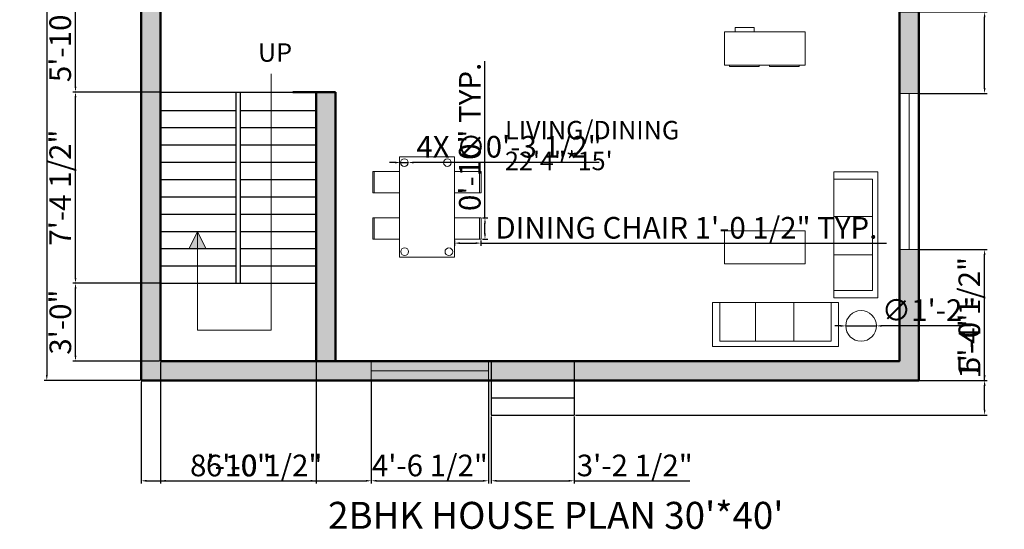
# Model space of a CAD drawing. Units: inches. Extents: x 1369 to 1956, y 3714 to 4363.
# Tile 1 of 2: x 1369 to 1825, y 3714 to 3949. Entities that reach past the tile are written whole.
import ezdxf

# ---------------------------------------------------------------- set-up
doc = ezdxf.new("R2010")
doc.units = ezdxf.units.IN
for name, color, linetype, lineweight in [('A-ANNO-DIMS', 2, 'Continuous', 18), ('A-ANNO-SYMB', 7, 'Continuous', 18), ('A-ANNO-TEXT', 7, 'Continuous', 25), ('A-AREA-IDEN', 7, 'Continuous', 25), ('A-FLOR-STRS', 7, 'Continuous', 25), ('A-FURN', 8, 'Continuous', 18), ('A-GLAZ', 4, 'Continuous', 18), ('A-WALL', 7, 'Continuous', 50), ('A-WALL-PATT', 252, 'Continuous', 13)]:
    doc.layers.add(name, color=color, linetype=linetype, lineweight=lineweight)
doc.styles.get("Standard").update_dxf_attribs({"font": 'arial.ttf'})
doc.dimstyles.new('ISO-25', dxfattribs={"dimtxt": 10, "dimasz": 2.5, "dimexe": 1.25, "dimexo": 0.625, "dimtad": 1, "dimdec": 0, "dimlunit": 4, "dimtxsty": 'Standard', "dimcen": 2.5, "dimadec": 0, "dimazin": 0, "dimtfac": 1, "dimtdec": 0, "dimtmove": 0, "dimatfit": 3, "dimfxl": 1, "dimarcsym": 0})

# ---------------------------------------------------------------- blocks, each defined once
blk = doc.blocks.new('*D6')
at = {"layer": 'A-ANNO-DIMS', "color": 0, "lineweight": -2, "transparency": 16777216}
for p, q in [((1424.56, 4262.45), (1380.24, 4262.45)), ((1381.49, 4259.95), (1381.49, 3784.95)), ((1424.56, 3782.45), (1380.24, 3782.45))]:
    blk.add_line(p, q, dxfattribs=at)
at = {"layer": 'A-ANNO-DIMS', "color": 0, "transparency": 16777216}
for points in [[(1381.07, 4259.95), (1381.9, 4259.95), (1381.49, 4262.45)], [(1381.07, 3784.95), (1381.9, 3784.95), (1381.49, 3782.45)]]:
    blk.add_solid(points, dxfattribs=at)
at = {"layer": 'Defpoints', "color": 0, "transparency": 16777216}
for p in [(1425.18, 4262.45), (1381.49, 3782.45), (1425.18, 3782.45)]:
    blk.add_point(p, dxfattribs=at)
at = {"layer": 'A-ANNO-DIMS', "color": 0, "transparency": 16777216, "insert": (1375.76, 4022.45), "char_height": 10, "attachment_point": 5, "rotation": 90}
blk.add_mtext("40'", dxfattribs=at)
blk = doc.blocks.new('WINDOW-72IN')
blk.add_line((0, 4.5), (72.22, 4.5))
blk.add_lwpolyline([(0, 9), (72.22, 9), (72.22, 0), (0, 0)], close=True)
blk = doc.blocks.new('CHAIR-DINING')
blk.add_line((11.59, 9.82), (11.59, 0))
blk.add_lwpolyline([(0, 9.82), (12.29, 9.82), (12.29, 0), (0, 0)], close=True)
blk = doc.blocks.new('*D12')
at = {"layer": 'A-ANNO-DIMS', "color": 0, "lineweight": -2, "transparency": 16777216}
for p, q in [((1570.19, 3847.22), (1570.19, 3844.76)), ((1582.47, 3847.22), (1582.47, 3844.76)), ((1572.69, 3846.01), (1579.97, 3846.01)), ((1582.47, 3846.01), (1770.1, 3846.01))]:
    blk.add_line(p, q, dxfattribs=at)
at = {"layer": 'A-ANNO-DIMS', "color": 0, "transparency": 16777216}
for points in [[(1572.69, 3846.42), (1572.69, 3845.59), (1570.19, 3846.01)], [(1579.97, 3846.42), (1579.97, 3845.59), (1582.47, 3846.01)]]:
    blk.add_solid(points, dxfattribs=at)
at = {"layer": 'Defpoints', "color": 0, "transparency": 16777216}
for p in [(1570.19, 3847.85), (1582.47, 3847.85), (1582.47, 3846.01)]:
    blk.add_point(p, dxfattribs=at)
at = {"layer": 'A-ANNO-DIMS', "color": 0, "transparency": 16777216, "insert": (1677.54, 3851.8), "char_height": 10, "attachment_point": 5}
blk.add_mtext('DINING CHAIR 1\'-0 1/2" TYP.', dxfattribs=at)
blk = doc.blocks.new('*D13')
at = {"layer": 'A-ANNO-DIMS', "color": 0, "lineweight": -2, "transparency": 16777216}
for p, q in [((1584.31, 3857.67), (1584.31, 3930.14)), ((1583.1, 3857.67), (1585.56, 3857.67)), ((1584.31, 3850.35), (1584.31, 3855.17)), ((1583.1, 3847.85), (1585.56, 3847.85))]:
    blk.add_line(p, q, dxfattribs=at)
at = {"layer": 'A-ANNO-DIMS', "color": 0, "transparency": 16777216}
for points in [[(1583.9, 3855.17), (1584.73, 3855.17), (1584.31, 3857.67)], [(1583.9, 3850.35), (1584.73, 3850.35), (1584.31, 3847.85)]]:
    blk.add_solid(points, dxfattribs=at)
at = {"layer": 'Defpoints', "color": 0, "transparency": 16777216}
for p in [(1582.47, 3857.67), (1584.31, 3857.67), (1582.47, 3847.85)]:
    blk.add_point(p, dxfattribs=at)
at = {"layer": 'A-ANNO-DIMS', "color": 0, "transparency": 16777216, "insert": (1578.58, 3895.16), "char_height": 10, "attachment_point": 5, "rotation": 90}
blk.add_mtext('0\'-10" TYP.', dxfattribs=at)
blk = doc.blocks.new('*D16')
at = {"layer": 'A-ANNO-DIMS', "color": 0, "lineweight": -2, "transparency": 16777216}
for p, q in [((1434.18, 3790.82), (1434.18, 3734.8)), ((1506.18, 3790.82), (1506.18, 3734.8)), ((1436.68, 3736.05), (1503.68, 3736.05))]:
    blk.add_line(p, q, dxfattribs=at)
at = {"layer": 'A-ANNO-DIMS', "color": 0, "transparency": 16777216}
for points in [[(1436.68, 3736.46), (1436.68, 3735.63), (1434.18, 3736.05)], [(1503.68, 3736.46), (1503.68, 3735.63), (1506.18, 3736.05)]]:
    blk.add_solid(points, dxfattribs=at)
at = {"layer": 'Defpoints', "color": 0, "transparency": 16777216}
for p in [(1434.18, 3791.45), (1506.18, 3791.45), (1506.18, 3736.05)]:
    blk.add_point(p, dxfattribs=at)
at = {"layer": 'A-ANNO-DIMS', "color": 0, "transparency": 16777216, "insert": (1470.18, 3741.78), "char_height": 10, "attachment_point": 5}
blk.add_mtext('6\'-0"', dxfattribs=at)
blk = doc.blocks.new('*D17')
at = {"layer": 'A-ANNO-DIMS', "color": 0, "lineweight": -2, "transparency": 16777216}
for p, q in [((1433.56, 3827.45), (1393.53, 3827.45)), ((1394.78, 3793.95), (1394.78, 3824.95)), ((1433.56, 3791.45), (1393.53, 3791.45))]:
    blk.add_line(p, q, dxfattribs=at)
at = {"layer": 'A-ANNO-DIMS', "color": 0, "transparency": 16777216}
for points in [[(1394.36, 3824.95), (1395.2, 3824.95), (1394.78, 3827.45)], [(1394.36, 3793.95), (1395.2, 3793.95), (1394.78, 3791.45)]]:
    blk.add_solid(points, dxfattribs=at)
at = {"layer": 'Defpoints', "color": 0, "transparency": 16777216}
for p in [(1394.78, 3827.45), (1434.18, 3827.45), (1434.18, 3791.45)]:
    blk.add_point(p, dxfattribs=at)
at = {"layer": 'A-ANNO-DIMS', "color": 0, "transparency": 16777216, "insert": (1389.05, 3809.45), "char_height": 10, "attachment_point": 5, "rotation": 90}
blk.add_mtext('3\'-0"', dxfattribs=at)
blk = doc.blocks.new('*D18')
at = {"layer": 'A-ANNO-DIMS', "color": 0, "lineweight": -2, "transparency": 16777216}
for p, q in [((1433.56, 3915.93), (1393.53, 3915.93)), ((1394.78, 3829.95), (1394.78, 3913.43)), ((1433.56, 3827.45), (1393.53, 3827.45))]:
    blk.add_line(p, q, dxfattribs=at)
at = {"layer": 'A-ANNO-DIMS', "color": 0, "transparency": 16777216}
for points in [[(1394.36, 3913.43), (1395.2, 3913.43), (1394.78, 3915.93)], [(1394.36, 3829.95), (1395.2, 3829.95), (1394.78, 3827.45)]]:
    blk.add_solid(points, dxfattribs=at)
at = {"layer": 'Defpoints', "color": 0, "transparency": 16777216}
for p in [(1394.78, 3915.93), (1434.18, 3915.93), (1434.18, 3827.45)]:
    blk.add_point(p, dxfattribs=at)
at = {"layer": 'A-ANNO-DIMS', "color": 0, "transparency": 16777216, "insert": (1388.99, 3871.69), "char_height": 10, "attachment_point": 5, "rotation": 90}
blk.add_mtext('7\'-4 1/2"', dxfattribs=at)
blk = doc.blocks.new('*D19')
at = {"layer": 'A-ANNO-DIMS', "color": 0, "lineweight": -2, "transparency": 16777216}
for p, q in [((1587.22, 3765.82), (1587.22, 3734.8)), ((1625.58, 3765.82), (1625.58, 3734.8)), ((1589.72, 3736.05), (1623.08, 3736.05)), ((1625.58, 3736.05), (1679.2, 3736.05))]:
    blk.add_line(p, q, dxfattribs=at)
at = {"layer": 'A-ANNO-DIMS', "color": 0, "transparency": 16777216}
for points in [[(1589.72, 3736.46), (1589.72, 3735.63), (1587.22, 3736.05)], [(1623.08, 3736.46), (1623.08, 3735.63), (1625.58, 3736.05)]]:
    blk.add_solid(points, dxfattribs=at)
at = {"layer": 'Defpoints', "color": 0, "transparency": 16777216}
for p in [(1587.22, 3766.45), (1625.58, 3766.45), (1625.58, 3736.05)]:
    blk.add_point(p, dxfattribs=at)
at = {"layer": 'A-ANNO-DIMS', "color": 0, "transparency": 16777216, "insert": (1653.64, 3741.85), "char_height": 10, "attachment_point": 5}
blk.add_mtext('3\'-2 1/2"', dxfattribs=at)
blk = doc.blocks.new('*D20')
at = {"layer": 'A-ANNO-DIMS', "color": 0, "lineweight": -2, "transparency": 16777216}
for p, q in [((1815.58, 3782.45), (1815.58, 3811.84)), ((1626.2, 3782.45), (1816.83, 3782.45)), ((1815.58, 3768.95), (1815.58, 3779.95)), ((1626.2, 3766.45), (1816.83, 3766.45))]:
    blk.add_line(p, q, dxfattribs=at)
at = {"layer": 'A-ANNO-DIMS', "color": 0, "transparency": 16777216}
for points in [[(1815.16, 3779.95), (1816, 3779.95), (1815.58, 3782.45)], [(1815.16, 3768.95), (1816, 3768.95), (1815.58, 3766.45)]]:
    blk.add_solid(points, dxfattribs=at)
at = {"layer": 'Defpoints', "color": 0, "transparency": 16777216}
for p in [(1625.58, 3782.45), (1815.58, 3782.45), (1625.58, 3766.45)]:
    blk.add_point(p, dxfattribs=at)
at = {"layer": 'A-ANNO-DIMS', "color": 0, "transparency": 16777216, "insert": (1809.94, 3798.39), "char_height": 10, "attachment_point": 5, "rotation": 90}
blk.add_mtext('1\'-4"', dxfattribs=at)
blk = doc.blocks.new('*D23')
at = {"layer": 'A-ANNO-DIMS', "color": 0, "lineweight": -2, "transparency": 16777216}
for p, q in [((1425.18, 3781.82), (1425.18, 3734.8)), ((1531.68, 3781.82), (1531.68, 3734.8)), ((1427.68, 3736.05), (1529.18, 3736.05))]:
    blk.add_line(p, q, dxfattribs=at)
at = {"layer": 'A-ANNO-DIMS', "color": 0, "transparency": 16777216}
for points in [[(1427.68, 3736.46), (1427.68, 3735.63), (1425.18, 3736.05)], [(1529.18, 3736.46), (1529.18, 3735.63), (1531.68, 3736.05)]]:
    blk.add_solid(points, dxfattribs=at)
at = {"layer": 'Defpoints', "color": 0, "transparency": 16777216}
for p in [(1425.18, 3782.45), (1531.68, 3782.45), (1531.68, 3736.05)]:
    blk.add_point(p, dxfattribs=at)
at = {"layer": 'A-ANNO-DIMS', "color": 0, "transparency": 16777216, "insert": (1478.43, 3741.84), "char_height": 10, "attachment_point": 5}
blk.add_mtext('8\'-10 1/2"', dxfattribs=at)
blk = doc.blocks.new('*D24')
at = {"layer": 'A-ANNO-DIMS', "color": 0, "lineweight": -2, "transparency": 16777216}
for p, q in [((1531.68, 3781.82), (1531.68, 3734.8)), ((1585.94, 3781.82), (1585.94, 3734.8)), ((1534.18, 3736.05), (1583.44, 3736.05))]:
    blk.add_line(p, q, dxfattribs=at)
at = {"layer": 'A-ANNO-DIMS', "color": 0, "transparency": 16777216}
for points in [[(1534.18, 3736.46), (1534.18, 3735.63), (1531.68, 3736.05)], [(1583.44, 3736.46), (1583.44, 3735.63), (1585.94, 3736.05)]]:
    blk.add_solid(points, dxfattribs=at)
at = {"layer": 'Defpoints', "color": 0, "transparency": 16777216}
for p in [(1531.68, 3782.45), (1585.94, 3782.45), (1585.94, 3736.05)]:
    blk.add_point(p, dxfattribs=at)
at = {"layer": 'A-ANNO-DIMS', "color": 0, "transparency": 16777216, "insert": (1558.81, 3741.84), "char_height": 10, "attachment_point": 5}
blk.add_mtext('4\'-6 1/2"', dxfattribs=at)
blk = doc.blocks.new('*D25')
at = {"layer": 'A-ANNO-DIMS', "color": 0, "lineweight": -2, "transparency": 16777216}
for p, q in [((1785.81, 3843.04), (1816.83, 3843.04)), ((1815.58, 3784.95), (1815.58, 3840.54)), ((1785.81, 3782.45), (1816.83, 3782.45))]:
    blk.add_line(p, q, dxfattribs=at)
at = {"layer": 'A-ANNO-DIMS', "color": 0, "transparency": 16777216}
for points in [[(1815.16, 3840.54), (1816, 3840.54), (1815.58, 3843.04)], [(1815.16, 3784.95), (1816, 3784.95), (1815.58, 3782.45)]]:
    blk.add_solid(points, dxfattribs=at)
at = {"layer": 'Defpoints', "color": 0, "transparency": 16777216}
for p in [(1785.18, 3843.04), (1815.58, 3843.04), (1785.18, 3782.45)]:
    blk.add_point(p, dxfattribs=at)
at = {"layer": 'A-ANNO-DIMS', "color": 0, "transparency": 16777216, "insert": (1809.79, 3812.74), "char_height": 10, "attachment_point": 5, "rotation": 90}
blk.add_mtext('5\'-0 1/2"', dxfattribs=at)
blk = doc.blocks.new('*D26')
at = {"layer": 'A-ANNO-DIMS', "color": 0, "lineweight": -2, "transparency": 16777216}
for p, q in [((1815.58, 3952.95), (1815.58, 4006.57)), ((1776.81, 3952.95), (1816.83, 3952.95)), ((1815.58, 3917.75), (1815.58, 3950.45)), ((1785.81, 3915.25), (1816.83, 3915.25))]:
    blk.add_line(p, q, dxfattribs=at)
at = {"layer": 'A-ANNO-DIMS', "color": 0, "transparency": 16777216}
for points in [[(1815.16, 3950.45), (1816, 3950.45), (1815.58, 3952.95)], [(1815.16, 3917.75), (1816, 3917.75), (1815.58, 3915.25)]]:
    blk.add_solid(points, dxfattribs=at)
at = {"layer": 'Defpoints', "color": 0, "transparency": 16777216}
for p in [(1776.18, 3952.95), (1815.58, 3952.95), (1785.18, 3915.25)]:
    blk.add_point(p, dxfattribs=at)
at = {"layer": 'A-ANNO-DIMS', "color": 0, "transparency": 16777216, "insert": (1809.78, 3981.01), "char_height": 10, "attachment_point": 5, "rotation": 90}
blk.add_mtext('3\'-1 1/2"', dxfattribs=at)
blk = doc.blocks.new('*D32')
at = {"layer": 'A-ANNO-DIMS', "color": 0, "lineweight": -2, "transparency": 16777216}
for p, q in [((1424.56, 3986.35), (1393.53, 3986.35)), ((1394.78, 3918.43), (1394.78, 3983.85)), ((1433.56, 3915.93), (1393.53, 3915.93))]:
    blk.add_line(p, q, dxfattribs=at)
at = {"layer": 'A-ANNO-DIMS', "color": 0, "transparency": 16777216}
for points in [[(1394.36, 3983.85), (1395.2, 3983.85), (1394.78, 3986.35)], [(1394.36, 3918.43), (1395.2, 3918.43), (1394.78, 3915.93)]]:
    blk.add_solid(points, dxfattribs=at)
at = {"layer": 'Defpoints', "color": 0, "transparency": 16777216}
for p in [(1394.78, 3986.35), (1425.18, 3986.35), (1434.18, 3915.93)]:
    blk.add_point(p, dxfattribs=at)
at = {"layer": 'A-ANNO-DIMS', "color": 0, "transparency": 16777216, "insert": (1388.99, 3951.14), "char_height": 10, "attachment_point": 5, "rotation": 90}
blk.add_mtext('5\'-10 1/2"', dxfattribs=at)
blk = doc.blocks.new('*D37')
at = {"layer": 'A-ANNO-DIMS', "color": 0, "lineweight": -2, "transparency": 16777216}
for p, q in [((1542.69, 3883.29), (1540.19, 3883.29)), ((1545.19, 3883.29), (1548.76, 3883.29)), ((1637.13, 3883.28), (1551.26, 3883.29))]:
    blk.add_line(p, q, dxfattribs=at)
at = {"layer": 'A-ANNO-DIMS', "color": 0, "transparency": 16777216}
for points in [[(1542.69, 3883.71), (1542.69, 3882.88), (1545.19, 3883.29)], [(1551.26, 3883.71), (1551.26, 3882.88), (1548.76, 3883.29)]]:
    blk.add_solid(points, dxfattribs=at)
at = {"layer": 'Defpoints', "color": 0, "transparency": 16777216}
for p in [(1545.19, 3883.29), (1548.76, 3883.29)]:
    blk.add_point(p, dxfattribs=at)
at = {"layer": 'A-ANNO-DIMS', "color": 0, "transparency": 16777216, "insert": (1595.44, 3889.3), "char_height": 10, "attachment_point": 5, "rotation": 359.9935}
blk.add_mtext('4X ∅0\'-3 1/2"', dxfattribs=at)
blk = doc.blocks.new('*D38')
at = {"layer": 'A-ANNO-DIMS', "color": 0, "lineweight": -2, "transparency": 16777216}
for p, q in [((1748.81, 3807.71), (1746.31, 3807.71)), ((1751.31, 3807.71), (1765.47, 3807.71)), ((1809.19, 3807.71), (1767.97, 3807.71))]:
    blk.add_line(p, q, dxfattribs=at)
at = {"layer": 'A-ANNO-DIMS', "color": 0, "transparency": 16777216}
for points in [[(1748.81, 3808.13), (1748.81, 3807.29), (1751.31, 3807.71)], [(1767.97, 3808.13), (1767.97, 3807.29), (1765.47, 3807.71)]]:
    blk.add_solid(points, dxfattribs=at)
at = {"layer": 'Defpoints', "color": 0, "transparency": 16777216}
for p in [(1751.31, 3807.71), (1765.47, 3807.71)]:
    blk.add_point(p, dxfattribs=at)
at = {"layer": 'A-ANNO-DIMS', "color": 0, "transparency": 16777216, "insert": (1789.83, 3813.72), "char_height": 10, "attachment_point": 5, "rotation": 359.9967}
blk.add_mtext('∅1\'-2"', dxfattribs=at)

msp = doc.modelspace()

# ---------------------------------------------------------------- hatches: boundary and pattern name
at = {"layer": 'A-ANNO-SYMB'}
h = msp.add_hatch(color=256, dxfattribs=at)
h.dxf.hatch_style = 1
h.paths.add_polyline_path([(1451.25, 3851.45), (1447.34, 3843.45), (1451.25, 3843.45)])
h.paths.add_polyline_path([(1451.25, 3851.45), (1451.25, 3843.45), (1455.17, 3843.45)])
at = {"layer": 'A-WALL-PATT'}
h = msp.add_hatch(color=256, dxfattribs=at)
h.dxf.hatch_style = 1
h.paths.add_polyline_path([(1785.18, 3997.53), (1776.18, 3997.53), (1776.18, 3915.25), (1785.18, 3915.25)])
h.paths.add_polyline_path([(1776.18, 3957.45), (1651.18, 3957.45), (1651.18, 3962.45), (1651.15, 3962.45), (1646.68, 3962.45), (1646.68, 3957.45), (1646.68, 3952.95), (1776.18, 3952.95)], flags=17)
h.paths.add_polyline_path([(1651.18, 4116.95), (1646.68, 4116.95), (1646.68, 3992.23), (1651.18, 3992.23)])
h.paths.add_polyline_path([(1585.18, 3957.45), (1434.18, 3957.45), (1434.18, 3952.95), (1582.18, 3952.95), (1585.18, 3952.95)], flags=17)
h.paths.add_polyline_path([(1434.18, 3986.35), (1425.18, 3986.35), (1425.18, 3782.45), (1785.18, 3782.45), (1785.18, 3843.04), (1776.18, 3843.04), (1776.18, 3791.45), (1434.18, 3791.45)])
h.paths.add_polyline_path([(1531.68, 4070.96), (1527.18, 4070.96), (1527.18, 4052.95), (1434.18, 4052.95), (1434.18, 4048.45), (1531.68, 4048.45)])
h.paths.add_polyline_path([(1434.18, 4048.45), (1434.18, 4052.95), (1434.18, 4068.61), (1425.18, 4068.61), (1425.18, 4028.64), (1434.18, 4028.64)])
h.paths.add_polyline_path([(1785.18, 4262.45), (1425.18, 4262.45), (1425.18, 4100.25), (1434.18, 4100.25), (1434.18, 4116.95), (1434.18, 4253.45), (1776.18, 4253.45), (1776.18, 4069.75), (1785.18, 4069.75)])
h.paths.add_polyline_path([(1776.18, 4121.45), (1651.18, 4121.45), (1651.18, 4116.95), (1776.18, 4116.95)], flags=17)
h.paths.add_polyline_path([(1651.18, 4121.45), (1646.68, 4121.45), (1646.68, 4116.95), (1651.18, 4116.95)], flags=17)
h.paths.add_polyline_path([(1582.68, 4125.18), (1578.18, 4125.18), (1578.18, 4121.45), (1434.18, 4121.45), (1434.18, 4116.95), (1582.68, 4116.95)], flags=17)
h.paths.add_polyline_path([(1582.68, 4253.45), (1578.18, 4253.45), (1578.18, 4154.96), (1578.21, 4154.96), (1582.68, 4154.96)], flags=17)
h.paths.add_polyline_path([(1651.18, 4253.45), (1646.68, 4253.45), (1646.68, 4193.53), (1646.71, 4193.53), (1651.18, 4193.53)], flags=17)
h.paths.add_polyline_path([(1646.68, 4160.45), (1582.68, 4160.45), (1582.68, 4155.95), (1646.68, 4155.95)], flags=17)
h.paths.add_polyline_path([(1651.18, 4163.74), (1646.68, 4163.74), (1646.68, 4160.45), (1646.68, 4155.95), (1651.18, 4155.95)], flags=17)
h.paths.add_polyline_path([(1651.18, 4123.87), (1646.68, 4123.87), (1646.68, 4121.45), (1651.18, 4121.45)], flags=17)
h.paths.add_polyline_path([(1651.18, 4155.95), (1646.68, 4155.95), (1646.68, 4153.66), (1651.18, 4153.66)], flags=17)
h.paths.add_polyline_path([(1515.18, 3904.98), (1515.18, 3915.93), (1506.18, 3915.93), (1506.18, 3894.63), (1506.18, 3791.45), (1515.18, 3791.45)], flags=17)

# ---------------------------------------------------------------- linework, layer by layer
at = {"layer": 'A-ANNO-SYMB'}
for p, q in [((1485.3, 3924.31), (1485.3, 3805.75)), ((1451.25, 3851.45), (1447.34, 3843.45)), ((1451.25, 3805.75), (1451.25, 3851.45)), ((1451.25, 3851.45), (1455.17, 3843.45)), ((1485.3, 3805.75), (1451.25, 3805.75))]:
    msp.add_line(p, q, dxfattribs=at)
at = {"layer": 'A-FLOR-STRS'}
for p, q in [((1434.18, 3915.93), (1506.18, 3915.93)), ((1469.18, 3827.45), (1469.18, 3915.93)), ((1471.18, 3827.45), (1471.18, 3915.93)), ((1434.18, 3907.45), (1469.18, 3907.45)), ((1471.18, 3907.45), (1506.18, 3907.45)), ((1434.18, 3899.45), (1469.18, 3899.45)), ((1471.18, 3899.45), (1506.18, 3899.45)), ((1434.18, 3891.45), (1469.18, 3891.45)), ((1471.18, 3891.45), (1506.18, 3891.45)), ((1434.18, 3883.45), (1469.18, 3883.45)), ((1471.18, 3883.45), (1506.18, 3883.45)), ((1434.18, 3875.45), (1469.18, 3875.45)), ((1471.18, 3875.45), (1506.18, 3875.45)), ((1434.18, 3867.45), (1469.18, 3867.45)), ((1471.18, 3867.45), (1506.18, 3867.45)), ((1434.18, 3859.45), (1469.18, 3859.45)), ((1471.18, 3859.45), (1506.18, 3859.45)), ((1434.18, 3851.45), (1469.18, 3851.45)), ((1471.18, 3851.45), (1506.18, 3851.45)), ((1434.18, 3843.45), (1469.18, 3843.45)), ((1471.18, 3843.45), (1506.18, 3843.45)), ((1434.18, 3835.45), (1469.18, 3835.45)), ((1471.18, 3835.45), (1506.18, 3835.45)), ((1434.18, 3827.45), (1506.18, 3827.45)), ((1587.22, 3791.45), (1587.22, 3766.45)), ((1625.58, 3791.45), (1625.58, 3766.45)), ((1587.22, 3782.45), (1625.58, 3782.45)), ((1587.22, 3774.45), (1625.58, 3774.45)), ((1587.22, 3766.45), (1625.58, 3766.45))]:
    msp.add_line(p, q, dxfattribs=at)
at = {"layer": 'A-FURN'}
for p, q in [((1766.21, 3878.99), (1745.86, 3878.99)), ((1745.86, 3875.62), (1745.86, 3878.99)), ((1766.21, 3820.63), (1766.21, 3878.99)), ((1763.69, 3858.27), (1745.86, 3858.27)), ((1763.69, 3840.54), (1745.86, 3840.54)), ((1745.86, 3820.63), (1766.21, 3820.63)), ((1689.57, 3818.52), (1689.57, 3798.18)), ((1709.48, 3800.69), (1709.48, 3818.52)), ((1727.21, 3800.69), (1727.21, 3818.52)), ((1747.93, 3818.52), (1741.5, 3818.52)), ((1747.93, 3798.18), (1747.93, 3818.52)), ((1689.57, 3798.18), (1747.93, 3798.18))]:
    msp.add_line(p, q, dxfattribs=at)
for points in [[(1732.57, 3928.33), (1695.25, 3928.33), (1695.25, 3943.71), (1732.57, 3943.71)], [(1700.16, 3943.71), (1708.87, 3943.71), (1708.87, 3945.82), (1700.16, 3945.82)], [(1697.45, 3928.33), (1711.17, 3928.33), (1711.17, 3927.66), (1697.45, 3927.66)], [(1715.96, 3928.33), (1729.68, 3928.33), (1729.68, 3927.66), (1715.96, 3927.66)], [(1544.67, 3839.57), (1570.19, 3839.57), (1570.19, 3885.93), (1544.67, 3885.93)], [(1763.69, 3875.62), (1763.69, 3824.06), (1745.86, 3824.06), (1745.86, 3875.62)], [(1732.57, 3836.37), (1695.25, 3836.37), (1695.25, 3851.75), (1732.57, 3851.75)], [(1745.86, 3824.06), (1745.86, 3820.63), (1745.86, 3820.63), (1745.86, 3824.06)], [(1693.01, 3818.52), (1689.57, 3818.52), (1689.57, 3818.52), (1693.01, 3818.52)], [(1744.57, 3800.69), (1693.01, 3800.69), (1693.01, 3818.52), (1744.57, 3818.52)]]:
    msp.add_lwpolyline(points, close=True, dxfattribs=at)
for centre, radius in [((1546.97, 3883.29), 1.78), ((1566.92, 3883.29), 1.78), ((1547.14, 3842.08), 1.78), ((1567.59, 3842.03), 1.78), ((1758.39, 3807.71), 7.08)]:
    msp.add_circle(centre, radius, dxfattribs=at)
at = {"layer": 'A-GLAZ'}
msp.add_line((1531.68, 3786.95), (1585.94, 3786.95), dxfattribs=at)
msp.add_lwpolyline([(1531.68, 3782.45), (1585.94, 3782.45), (1585.94, 3791.45), (1531.68, 3791.45)], close=True, dxfattribs=at)
at = {"layer": 'A-WALL'}
for p, q in [((1515.18, 3915.93), (1495.31, 3915.93)), ((1506.18, 3915.93), (1506.18, 3894.63)), ((1515.18, 3904.98), (1515.18, 3915.93)), ((1506.18, 3791.45), (1506.18, 3904.98)), ((1515.18, 3791.45), (1515.18, 3904.98)), ((1434.18, 3791.45), (1434.18, 3827.45)), ((1434.18, 3791.45), (1506.18, 3791.45))]:
    msp.add_line(p, q, dxfattribs=at)
for points in [[(1425.18, 3782.45), (1785.18, 3782.45), (1785.18, 4262.45), (1425.18, 4262.45)], [(1434.18, 3791.45), (1776.18, 3791.45), (1776.18, 4253.45), (1434.18, 4253.45)]]:
    msp.add_lwpolyline(points, close=True, dxfattribs=at)

# ---------------------------------------------------------------- block references
at = {"layer": 'A-FURN', "extrusion": (0, 0, -1), "zscale": -1}
for p in [(-1544.67, 3869.33), (-1544.67, 3847.85)]:
    msp.add_blockref('CHAIR-DINING', p, dxfattribs=at)
at = {"layer": 'A-FURN'}
for p in [(1570.19, 3869.33), (1570.19, 3847.85)]:
    msp.add_blockref('CHAIR-DINING', p, dxfattribs=at)
at = {"layer": 'A-GLAZ', "rotation": 269.9999999999998}
msp.add_blockref('WINDOW-72IN', (1776.18, 3915.25), dxfattribs=at)

# ---------------------------------------------------------------- texts
at = {"layer": 'A-ANNO-TEXT', "attachment_point": 1}
for s, width, gutter_width, insert, char_height in [('UP', 219.0068, 42.75, (1479.25, 3938.47), 8.55), ("2BHK HOUSE PLAN 30'*40'", 1556.6621, 62.39, (1511.67, 3726.3), 12.4783)]:
    msp.add_mtext_dynamic_manual_height_columns(s, width=width, gutter_width=gutter_width, heights=[0], dxfattribs=dict(at, insert=insert, char_height=char_height))
at = {"layer": 'A-AREA-IDEN', "insert": (1593.56, 3902.56), "char_height": 8.5497, "attachment_point": 1}
msp.add_mtext_dynamic_manual_height_columns('LIVING/DINING\\P22\'4"*15\'', width=219.0068, gutter_width=42.75, heights=[0], dxfattribs=at)

# ---------------------------------------------------------------- dimensions: what is measured, and where the dimension line sits
at = {"layer": 'A-ANNO-DIMS'}
for base, p1, p2, override, picture, middle in [((1381.49, 3782.45), (1425.18, 4262.45), (1425.18, 3782.45), {"dimclrd": 0, "dimclre": 0, "dimclrt": 0}, '*D6', (1375.76, 4022.45)), ((1815.58, 3952.95), (1785.18, 3915.25), (1776.18, 3952.95), {"dimdec": 1, "dimlfac": 1, "dimrnd": 0, "dimzin": 1, "dimdsep": 46, "dimlunit": 4, "dimfrac": 2}, '*D26', (1809.78, 3981.01)), ((1394.78, 3986.35), (1434.18, 3915.93), (1425.18, 3986.35), {"dimdec": 1, "dimlfac": 1, "dimrnd": 0, "dimzin": 1, "dimdsep": 46, "dimlunit": 4, "dimfrac": 2}, '*D32', (1388.99, 3951.14)), ((1394.78, 3915.93), (1434.18, 3827.45), (1434.18, 3915.93), {"dimdec": 1, "dimlfac": 1, "dimrnd": 0, "dimzin": 1, "dimdsep": 46, "dimlunit": 4, "dimfrac": 2}, '*D18', (1388.99, 3871.69)), ((1815.58, 3843.04), (1785.18, 3782.45), (1785.18, 3843.04), {"dimdec": 1, "dimlfac": 1, "dimrnd": 0, "dimzin": 1, "dimdsep": 46, "dimlunit": 4, "dimfrac": 2}, '*D25', (1809.79, 3812.74)), ((1394.78, 3827.45), (1434.18, 3791.45), (1434.18, 3827.45), {"dimdec": 1, "dimlfac": 1, "dimrnd": 0, "dimzin": 1, "dimdsep": 46, "dimlunit": 4, "dimfrac": 2}, '*D17', (1389.05, 3809.45)), ((1815.58, 3782.45), (1625.58, 3766.45), (1625.58, 3782.45), {"dimdec": 1, "dimlfac": 1, "dimrnd": 0, "dimzin": 1, "dimdsep": 46, "dimlunit": 4, "dimfrac": 2}, '*D20', (1809.94, 3798.39))]:
    dim = msp.add_linear_dim(base=base, p1=p1, p2=p2, angle=90, dimstyle='ISO-25', override=override, dxfattribs=at)
    dim.commit()
    dim.dimension.update_dxf_attribs({"geometry": picture, "text_midpoint": middle})
dim = msp.add_linear_dim(base=(1584.31, 3857.67), p1=(1582.47, 3847.85), p2=(1582.47, 3857.67), angle=90, text='<> TYP.', dimstyle='ISO-25', override={"dimdec": 1, "dimlfac": 1, "dimrnd": 0, "dimzin": 1, "dimdsep": 46, "dimlunit": 4, "dimfrac": 2}, dxfattribs=at)
dim.commit()
dim.dimension.update_dxf_attribs({"geometry": '*D13', "text_midpoint": (1578.58, 3895.16)})
dim = msp.add_diameter_dim_2p(p1=(1545.19, 3883.29), p2=(1548.76, 3883.29), text='4X <>', dimstyle='ISO-25', override={"dimdec": 1, "dimlfac": 1, "dimrnd": 0, "dimzin": 1, "dimdsep": 46, "dimlunit": 4, "dimfrac": 2}, dxfattribs=at)
dim.commit()
dim.dimension.update_dxf_attribs({"geometry": '*D37', "text_midpoint": (1595.44, 3883.29), "dimtype": 163})
dim = msp.add_linear_dim(base=(1582.47, 3846.01), p1=(1570.19, 3847.85), p2=(1582.47, 3847.85), text='DINING CHAIR <> TYP.', dimstyle='ISO-25', override={"dimdec": 1, "dimlfac": 1, "dimrnd": 0, "dimzin": 1, "dimdsep": 46, "dimlunit": 4, "dimfrac": 2}, dxfattribs=at)
dim.commit()
dim.dimension.update_dxf_attribs({"geometry": '*D12', "text_midpoint": (1677.54, 3851.8)})
dim = msp.add_diameter_dim_2p(p1=(1751.31, 3807.71), p2=(1765.47, 3807.71), dimstyle='ISO-25', override={"dimdec": 1, "dimlfac": 1, "dimrnd": 0, "dimzin": 1, "dimdsep": 46, "dimlunit": 4, "dimfrac": 2}, dxfattribs=at)
dim.commit()
dim.dimension.update_dxf_attribs({"geometry": '*D38', "text_midpoint": (1789.83, 3807.71)})
for base, p1, p2, picture, middle in [((1506.18, 3736.05), (1434.18, 3791.45), (1506.18, 3791.45), '*D16', (1470.18, 3741.78)), ((1531.68, 3736.05), (1425.18, 3782.45), (1531.68, 3782.45), '*D23', (1478.43, 3741.84)), ((1585.94, 3736.05), (1531.68, 3782.45), (1585.94, 3782.45), '*D24', (1558.81, 3741.84)), ((1625.58, 3736.05), (1587.22, 3766.45), (1625.58, 3766.45), '*D19', (1653.64, 3741.85))]:
    dim = msp.add_linear_dim(base=base, p1=p1, p2=p2, dimstyle='ISO-25', override={"dimdec": 1, "dimlfac": 1, "dimrnd": 0, "dimzin": 1, "dimdsep": 46, "dimlunit": 4, "dimfrac": 2}, dxfattribs=at)
    dim.commit()
    dim.dimension.update_dxf_attribs({"geometry": picture, "text_midpoint": middle})

doc.saveas('drawing.dxf')
